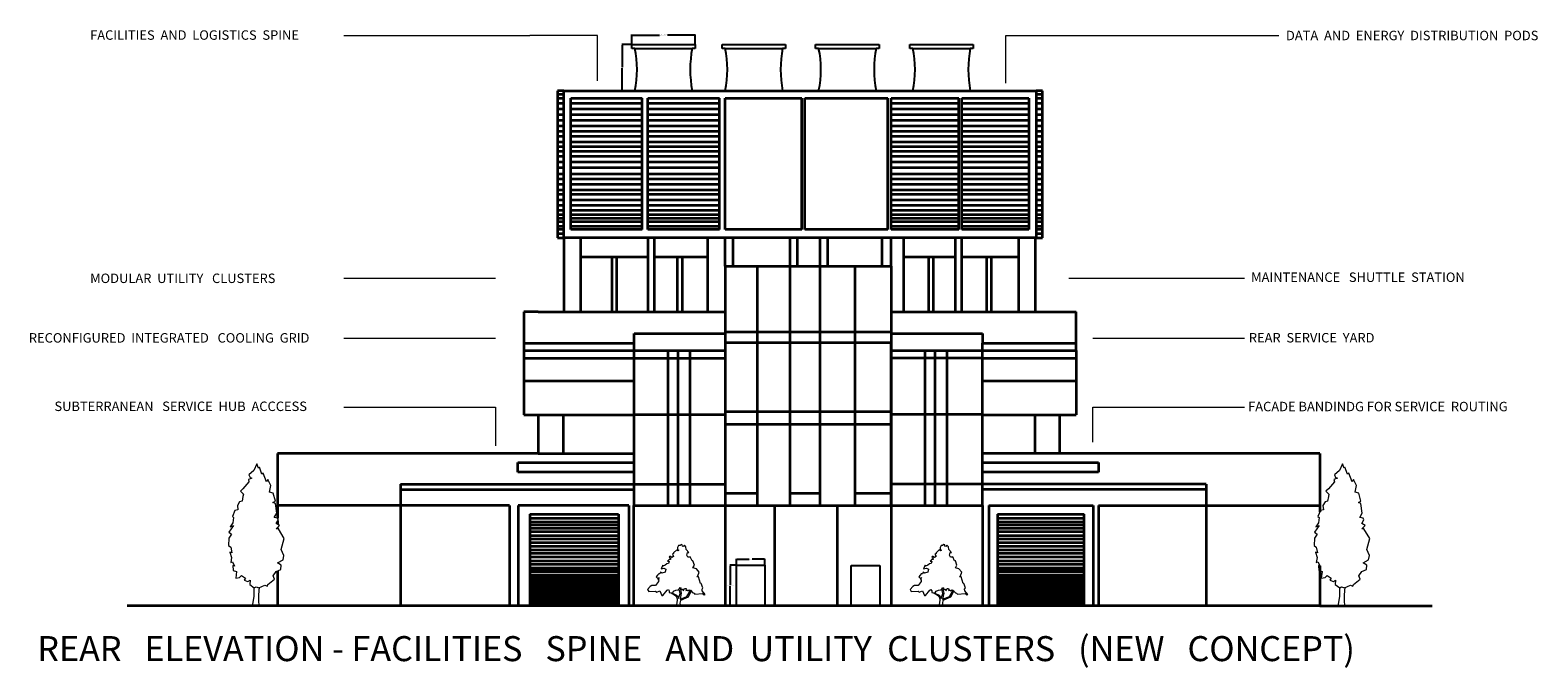
# Model space of a CAD drawing. Units: inches. Extents: x 13 to 584, y -20 to 222.
import ezdxf

# ---------------------------------------------------------------- set-up
doc = ezdxf.new("R2010")
doc.units = ezdxf.units.IN
doc.header["$MEASUREMENT"] = 0
for name, color, linetype, lineweight in [('A-ANNO-DIMS', 2, 'Continuous', 18), ('A-ANNO-SYMB', 2, 'Continuous', 18), ('A-ANNO-TEXT', 7, 'Continuous', 25), ('A-DOOR', 4, 'Continuous', 25), ('A-ELEV', 7, 'Continuous', 35), ('A-EQPM', 8, 'Continuous', 25), ('L-PLNT', 3, 'Continuous', 18)]:
    doc.layers.add(name, color=color, linetype=linetype, lineweight=lineweight)
doc.styles.get("Standard").update_dxf_attribs({"font": 'arial.ttf'})
doc.dimstyles.get("Standard").update_dxf_attribs({"dimtxt": 0.18, "dimasz": 0.18, "dimexe": 0.18, "dimexo": 0.0625, "dimgap": 0.09, "dimtad": 0, "dimtih": 1, "dimtoh": 1, "dimdec": 4, "dimzin": 0, "dimdsep": 46, "dimtxsty": 'Standard', "dimcen": 0.09, "dimadec": 0, "dimazin": 0, "dimtfac": 1, "dimtdec": 4, "dimtofl": 0, "dimtmove": 0, "dimatfit": 3, "dimfxl": 1, "dimtolj": 1, "dimtzin": 0, "dimarcsym": 0})

# ---------------------------------------------------------------- blocks, each defined once
blk = doc.blocks.new('*U2')
blk.add_lwpolyline([(-2.754, 191.699), (-6.78, 182.851), (-13.682, 176.953), (-11.956, 173.266), (-9.656, 172.529), (-14.257, 170.317), (-13.682, 167.368), (-21.733, 157.783), (-25.184, 154.834), (-21.158, 150.41), (-21.733, 147.461), (-22.884, 140.825), (-26.334, 140.087), (-29.21, 134.926), (-28.635, 129.028), (-32.661, 128.291), (-36.111, 120.18), (-34.386, 118.706), (-35.536, 111.333), (-38.987, 106.171), (-34.386, 107.646), (-40.712, 98.798), (-37.261, 95.849), (-40.712, 90.688), (-41.287, 80.366), (-38.412, 78.154), (-36.686, 70.781), (-39.562, 71.518), (-37.261, 64.145), (-38.412, 57.509), (-36.111, 58.247), (-33.236, 52.348), (-35.536, 53.086), (-34.961, 46.45), (-30.36, 44.975), (-31.51, 36.128), (-26.334, 36.865), (-23.459, 39.814), (-18.283, 36.128), (-20.008, 33.178), (-14.832, 31.704), (-11.956, 33.178), (-12.531, 27.28), (-6.205, 22.856), (-3.905, 24.331), (0.121, 22.856), (8.173, 26.543), (11.624, 25.068), (12.199, 27.28), (21.4, 34.653), (19.675, 39.077), (23.701, 44.975), (30.027, 47.924), (30.602, 53.823), (25.426, 56.772), (32.903, 61.196), (34.053, 67.094), (30.602, 75.205), (34.628, 89.951), (26.576, 103.222), (23.701, 103.222), (28.302, 107.646), (23.701, 110.595), (26.576, 115.756), (25.426, 117.968), (20.825, 118.706), (24.276, 124.604), (22.551, 137.876), (19.1, 139.35), (22.551, 140.825), (19.675, 151.884), (14.499, 153.359), (16.224, 162.207), (12.199, 170.317), (10.473, 167.368), (5.872, 179.165), (4.147, 177.69), (0.696, 187.275), (-0.454, 185.8)], close=True)
for points in [[(-6.813, 23.669), (-6.813, 11.669), (-8.627, 0)], [(0.387, 23.669), (-0.576, 13.271), (-0.576, 3.686), (0, 0)]]:
    blk.add_lwpolyline(points)
blk = doc.blocks.new('*U3')
for points in [[(22.0124, 137.721), (18.5475, 141.5624), (15.5282, 138.2446), (13.8028, 139.3505), (13.3714, 142.1153), (11.2148, 143.2214), (8.1954, 140.4564), (4.7447, 141.0094), (2.1567, 136.0326), (2.1567, 131.6088), (5.6074, 129.9499), (3.0193, 128.2909), (0.4313, 130.5029), (-6.9015, 123.3141), (-6.9015, 121.6552), (-9.9208, 119.9963), (-9.0581, 118.3373), (-6.9015, 115.0195), (-10.7835, 112.2546), (-14.6656, 115.0195), (-16.8222, 114.4665), (-17.6849, 112.2546), (-14.6656, 111.7016), (-14.2342, 107.2778), (-17.6065, 107.8307), (-21.5669, 103.9599), (-17.2536, 103.4069), (-18.9789, 97.8771), (-22.8609, 97.3241), (-27.1743, 94.5593), (-32.3504, 91.7944), (-32.7817, 94.0063), (-36.6638, 85.7116), (-29.7624, 87.3705), (-25.449, 84.6056), (-26.743, 77.9699), (-34.507, 75.205), (-37.9578, 77.4169), (-39.2518, 74.099), (-42.2711, 73.5461), (-44.8592, 70.2282), (-47.8786, 66.3574), (-43.9965, 63.0395), (-41.4085, 64.6985), (-44.3346, 59.8898), (-42.2089, 60.1377), (-42.5159, 55.7849), (-49.6039, 46.4502), (-58.2307, 45.8972), (-62.1127, 43.6853), (-68.5828, 36.4966), (-65.9947, 32.0727), (-50.0352, 32.6257), (-47.0159, 30.4138), (-39.6831, 33.7317), (-34.507, 22.6721), (-32.3504, 22.6721), (-22.4296, 34.8376), (-19.4102, 36.4966), (-17.2536, 33.7317), (-17.2536, 29.8608), (-13.8028, 28.7549), (-9.0581, 28.7549), (-7.3328, 32.6257), (-1.7254, 35.3906), (3.8821, 35.9436), (6.4701, 38.1555), (6.9014, 38.7085), (8.1954, 41.4734), (9.9208, 40.3674), (11.2148, 35.9436), (14.2341, 37.6025), (15.0968, 36.4966), (15.9595, 33.7317), (18.9789, 38.7085), (21.9982, 38.7085), (23.2922, 36.4966), (21.9982, 34.2847), (25.4489, 35.3906), (26.743, 33.7317), (29.7623, 35.9436), (32.7817, 34.8376), (38.8204, 28.7549), (41.4084, 27.6489), (43.5651, 25.437), (61.6813, 27.0959), (65.132, 23.7781), (67.7201, 24.884), (60.8186, 33.7317), (60.3873, 37.0495), (62.544, 40.3674), (58.662, 50.874), (56.5053, 50.874), (52.1919, 66.3574), (47.8785, 66.9103), (50.4665, 69.1222), (53.9172, 77.9699), (47.0158, 85.1586), (38.3891, 87.9235), (42.2711, 94.0063)], [(42.2711, 94.0063), (38.8204, 104.5129), (36.6637, 104.5129), (32.3503, 113.9135), (29.7623, 113.3605), (26.743, 113.3605), (24.5862, 117.7844), (25.8802, 123.8671), (29.331, 123.8671), (22.8609, 131.6088), (21.9982, 137.6916)], [(-9.9208, 28.2019), (0, 23.2251), (3.4507, 19.9072), (4.7447, 15.4834), (8.6267, 27.0959), (6.4701, 37.6025)], [(8.1954, 40.3674), (11.2148, 27.6489), (8.1954, 13.8245), (24.5862, 19.9072), (32.7817, 34.2847)], [(-12.9401, 28.7549), (-2.588, 22.1191), (0.8626, 17.6953), (1.7253, 11.6125), (0, 0)], [(34.5071, 33.1787), (27.1743, 18.2483), (9.0581, 10.5066), (7.7641, 3.8708), (8.1954, 0)]]:
    blk.add_lwpolyline(points)
blk = doc.blocks.new('COOLING-UNIT')
for p, q in [((0, 16.07), (0, 17.49)), ((0, 17.49), (24.03, 17.49)), ((24.03, 17.49), (24.03, 16.07)), ((1.14, 16.07), (0, 16.07)), ((1.14, 16.07), (22.88, 16.07)), ((24.03, 16.07), (22.88, 16.07))]:
    blk.add_line(p, q)
for centre, radius, start, end in [((-35.24, 8.04), 37.26, 347.5421, 12.4579), ((66.1, 8.04), 43.96, 169.4653, 190.5347)]:
    blk.add_arc(centre, radius, start, end)
blk = doc.blocks.new('DOOR-SERVICE')
for p, q in [((0, 0), (0, 15.29)), ((0, 15.29), (10.82, 15.29)), ((10.82, 15.29), (10.82, 0))]:
    blk.add_line(p, q)
blk = doc.blocks.new('*D6')
at = {"layer": 'A-ANNO-DIMS', "color": 0, "lineweight": -2, "transparency": 16777216}
for p, q in [((241.11, 216.34), (241.11, 220.06)), ((241.29, 219.88), (251.66, 219.88)), ((264.97, 219.88), (254.6, 219.88)), ((265.15, 216.34), (265.15, 220.06))]:
    blk.add_line(p, q, dxfattribs=at)
at = {"layer": 'A-ANNO-DIMS', "color": 0, "transparency": 16777216}
for points in [[(241.29, 219.91), (241.29, 219.85), (241.11, 219.88)], [(264.97, 219.91), (264.97, 219.85), (265.15, 219.88)]]:
    blk.add_solid(points, dxfattribs=at)
at = {"layer": 'Defpoints', "color": 0, "transparency": 16777216}
for p in [(265.15, 219.88), (241.11, 216.27), (265.15, 216.27)]:
    blk.add_point(p, dxfattribs=at)
at = {"layer": 'A-ANNO-DIMS', "color": 0, "transparency": 16777216, "insert": (253.13, 219.88), "char_height": 0.18, "attachment_point": 5}
blk.add_mtext('\\A1;COOLING UNIT 24 TYP.', dxfattribs=at)
blk = doc.blocks.new('*D7')
at = {"layer": 'A-ANNO-DIMS', "color": 0, "lineweight": -2, "transparency": 16777216}
for p, q in [((241.05, 216.27), (237.33, 216.27)), ((237.51, 216.09), (237.51, 207.71)), ((237.51, 198.96), (237.51, 207.35)), ((241.05, 198.78), (237.33, 198.78))]:
    blk.add_line(p, q, dxfattribs=at)
at = {"layer": 'A-ANNO-DIMS', "color": 0, "transparency": 16777216}
for points in [[(237.48, 216.09), (237.54, 216.09), (237.51, 216.27)], [(237.48, 198.96), (237.54, 198.96), (237.51, 198.78)]]:
    blk.add_solid(points, dxfattribs=at)
at = {"layer": 'Defpoints', "color": 0, "transparency": 16777216}
for p in [(237.51, 216.27), (241.11, 216.27), (241.11, 198.78)]:
    blk.add_point(p, dxfattribs=at)
at = {"layer": 'A-ANNO-DIMS', "color": 0, "transparency": 16777216, "insert": (237.51, 207.53), "char_height": 0.18, "attachment_point": 5}
blk.add_mtext('\\A1;17 TYP.', dxfattribs=at)
blk = doc.blocks.new('*D8')
at = {"layer": 'A-ANNO-DIMS', "color": 0, "lineweight": -2, "transparency": 16777216}
for p, q in [((280.67, 19.12), (278.26, 19.12)), ((278.44, 18.94), (278.44, 11.66)), ((278.44, 4.01), (278.44, 11.29)), ((280.67, 3.83), (278.26, 3.83))]:
    blk.add_line(p, q, dxfattribs=at)
at = {"layer": 'A-ANNO-DIMS', "color": 0, "transparency": 16777216}
for points in [[(278.41, 18.94), (278.47, 18.94), (278.44, 19.12)], [(278.41, 4.01), (278.47, 4.01), (278.44, 3.83)]]:
    blk.add_solid(points, dxfattribs=at)
at = {"layer": 'Defpoints', "color": 0, "transparency": 16777216}
for p in [(278.44, 19.12), (280.73, 19.12), (280.73, 3.83)]:
    blk.add_point(p, dxfattribs=at)
at = {"layer": 'A-ANNO-DIMS', "color": 0, "transparency": 16777216, "insert": (278.44, 11.47), "char_height": 0.18, "attachment_point": 5}
blk.add_mtext('\\A1;SERVICE DOOR 15 TYP.', dxfattribs=at)
blk = doc.blocks.new('*D9')
at = {"layer": 'A-ANNO-DIMS', "color": 0, "lineweight": -2, "transparency": 16777216}
for p, q in [((280.73, 19.18), (280.73, 21.59)), ((280.91, 21.41), (285.62, 21.41)), ((291.37, 21.41), (286.66, 21.41)), ((291.55, 19.18), (291.55, 21.59))]:
    blk.add_line(p, q, dxfattribs=at)
at = {"layer": 'A-ANNO-DIMS', "color": 0, "transparency": 16777216}
for points in [[(280.91, 21.44), (280.91, 21.38), (280.73, 21.41)], [(291.37, 21.44), (291.37, 21.38), (291.55, 21.41)]]:
    blk.add_solid(points, dxfattribs=at)
at = {"layer": 'Defpoints', "color": 0, "transparency": 16777216}
for p in [(280.73, 19.12), (291.55, 21.41), (291.55, 19.12)]:
    blk.add_point(p, dxfattribs=at)
at = {"layer": 'A-ANNO-DIMS', "color": 0, "transparency": 16777216, "insert": (286.14, 21.41), "char_height": 0.18, "attachment_point": 5}
blk.add_mtext('\\A1;11 TYP.', dxfattribs=at)

msp = doc.modelspace()

# ---------------------------------------------------------------- linework, layer by layer
at = {"layer": 'A-ANNO-SYMB'}
for p, q in [((132.16, 219.75), (202.59, 219.75)), ((228.21, 219.75), (202.59, 219.75)), ((228.21, 202.53), (228.21, 219.75)), ((382.77, 201.61), (382.77, 219.75)), ((382.77, 219.75), (486.08, 219.75)), ((132.16, 127.9), (189.57, 127.9)), ((406.56, 127.9), (473.06, 127.9)), ((132.16, 105.07), (189.57, 105.07)), ((415.65, 105.07), (473.06, 105.07)), ((132.16, 78.99), (189.57, 78.99)), ((189.57, 78.99), (189.57, 64.36)), ((415.65, 65.75), (415.65, 78.99)), ((415.65, 78.99), (473.06, 78.99))]:
    msp.add_line(p, q, dxfattribs=at)
at = {"layer": 'A-ELEV'}
for p, q in [((215.46, 198.78), (213.08, 198.78)), ((213.08, 198.78), (213.08, 143.13)), ((213.08, 197.55), (215.46, 197.55)), ((213.08, 195.94), (215.46, 195.94)), ((213.08, 194.05), (215.46, 194.05)), ((215.46, 198.78), (394.39, 198.78)), ((215.46, 143.13), (215.46, 198.78)), ((218.09, 195.94), (245.06, 195.94)), ((218.09, 146.31), (218.09, 195.94)), ((218.09, 194.05), (245.06, 194.05)), ((245.06, 146.31), (245.06, 195.94)), ((247.21, 195.94), (274.37, 195.94)), ((247.21, 146.31), (247.21, 195.94)), ((247.21, 194.05), (274.37, 194.05)), ((274.37, 146.31), (274.37, 195.94)), ((276.52, 195.94), (305.52, 195.94)), ((276.52, 146.31), (276.52, 195.94)), ((305.52, 146.31), (305.52, 195.94)), ((306.69, 195.94), (338.12, 195.94)), ((306.69, 146.31), (306.69, 195.94)), ((338.12, 146.31), (338.12, 195.94)), ((339.29, 195.94), (364.89, 195.94)), ((339.29, 146.31), (339.29, 195.94)), ((339.29, 194.05), (364.89, 194.05)), ((364.89, 146.31), (364.89, 195.94)), ((366.07, 195.94), (391.39, 195.94)), ((366.07, 146.31), (366.07, 195.94)), ((366.07, 194.05), (391.39, 194.05)), ((391.39, 195.94), (391.39, 146.31)), ((396.59, 198.78), (394.21, 198.78)), ((394.21, 198.78), (394.21, 143.13)), ((394.21, 197.55), (396.59, 197.55)), ((394.21, 195.94), (396.59, 195.94)), ((394.21, 194.05), (396.59, 194.05)), ((396.59, 143.13), (396.59, 198.78)), ((213.08, 191.91), (215.46, 191.91)), ((213.08, 189.77), (215.46, 189.77)), ((218.09, 191.91), (245.06, 191.91)), ((218.09, 189.77), (245.06, 189.77)), ((247.21, 191.91), (274.37, 191.91)), ((247.21, 189.77), (274.37, 189.77)), ((339.29, 191.91), (364.89, 191.91)), ((339.29, 189.77), (364.89, 189.77)), ((366.07, 191.91), (391.39, 191.91)), ((366.07, 189.77), (391.39, 189.77)), ((394.21, 191.91), (396.59, 191.91)), ((394.21, 189.77), (396.59, 189.77)), ((213.08, 187.63), (215.46, 187.63)), ((213.08, 185.49), (215.46, 185.49)), ((213.08, 183.54), (215.46, 183.54)), ((218.09, 187.63), (245.06, 187.63)), ((218.09, 185.49), (245.06, 185.49)), ((218.09, 183.54), (245.06, 183.54)), ((247.21, 187.63), (274.37, 187.63)), ((247.21, 185.49), (274.37, 185.49)), ((247.21, 183.54), (274.37, 183.54)), ((339.29, 187.63), (364.89, 187.63)), ((339.29, 185.49), (364.89, 185.49)), ((339.29, 183.54), (364.89, 183.54)), ((366.07, 187.63), (391.39, 187.63)), ((366.07, 185.49), (391.39, 185.49)), ((366.07, 183.54), (391.39, 183.54)), ((394.21, 187.63), (396.59, 187.63)), ((394.21, 185.49), (396.59, 185.49)), ((394.21, 183.54), (396.59, 183.54)), ((213.08, 181.6), (215.46, 181.6)), ((213.08, 179.46), (215.46, 179.46)), ((213.08, 177.71), (215.46, 177.71)), ((218.09, 181.6), (245.06, 181.6)), ((218.09, 179.46), (245.06, 179.46)), ((218.09, 177.71), (245.06, 177.71)), ((247.21, 181.6), (274.37, 181.6)), ((247.21, 179.46), (274.37, 179.46)), ((247.21, 177.71), (274.37, 177.71)), ((339.29, 181.6), (364.89, 181.6)), ((339.29, 179.46), (364.89, 179.46)), ((339.29, 177.71), (364.89, 177.71)), ((366.07, 181.6), (391.39, 181.6)), ((366.07, 179.46), (391.39, 179.46)), ((366.07, 177.71), (391.39, 177.71)), ((394.21, 181.6), (396.59, 181.6)), ((394.21, 179.46), (396.59, 179.46)), ((394.21, 177.71), (396.59, 177.71)), ((213.08, 175.96), (215.46, 175.96)), ((213.08, 174.01), (215.46, 174.01)), ((213.08, 171.85), (215.46, 171.85)), ((218.09, 175.96), (245.06, 175.96)), ((218.09, 174.01), (245.06, 174.01)), ((218.09, 171.85), (245.06, 171.85)), ((247.21, 175.96), (274.37, 175.96)), ((247.21, 174.01), (274.37, 174.01)), ((247.21, 171.85), (274.37, 171.85)), ((339.29, 175.96), (364.89, 175.96)), ((339.29, 174.01), (364.89, 174.01)), ((339.29, 171.85), (364.89, 171.85)), ((366.07, 175.96), (391.39, 175.96)), ((366.07, 174.01), (391.39, 174.01)), ((366.07, 171.85), (391.39, 171.85)), ((394.21, 175.96), (396.59, 175.96)), ((394.21, 174.01), (396.59, 174.01)), ((394.21, 171.85), (396.59, 171.85)), ((213.08, 169.71), (215.46, 169.71)), ((213.08, 167.37), (215.46, 167.37)), ((218.09, 169.71), (245.06, 169.71)), ((218.09, 167.37), (245.06, 167.37)), ((247.21, 169.71), (274.37, 169.71)), ((247.21, 167.37), (274.37, 167.37)), ((339.29, 169.71), (364.89, 169.71)), ((339.29, 167.37), (364.89, 167.37)), ((366.07, 169.71), (391.39, 169.71)), ((366.07, 167.37), (391.39, 167.37)), ((394.21, 169.71), (396.59, 169.71)), ((394.21, 167.37), (396.59, 167.37)), ((213.08, 165.43), (215.46, 165.43)), ((213.08, 163.48), (215.46, 163.48)), ((213.08, 161.34), (215.46, 161.34)), ((218.09, 165.43), (245.06, 165.43)), ((218.09, 163.48), (245.06, 163.48)), ((218.09, 161.34), (245.06, 161.34)), ((247.21, 165.43), (274.37, 165.43)), ((247.21, 163.48), (274.37, 163.48)), ((247.21, 161.34), (274.37, 161.34)), ((339.29, 165.43), (364.89, 165.43)), ((339.29, 163.48), (364.89, 163.48)), ((339.29, 161.34), (364.89, 161.34)), ((366.07, 165.43), (391.39, 165.43)), ((366.07, 163.48), (391.39, 163.48)), ((366.07, 161.34), (391.39, 161.34)), ((394.21, 165.43), (396.59, 165.43)), ((394.21, 163.48), (396.59, 163.48)), ((394.21, 161.34), (396.59, 161.34)), ((213.08, 159.59), (215.46, 159.59)), ((213.08, 157.45), (215.46, 157.45)), ((213.08, 155.51), (215.46, 155.51)), ((218.09, 159.59), (245.06, 159.59)), ((218.09, 157.45), (245.06, 157.45)), ((218.09, 155.51), (245.06, 155.51)), ((247.21, 159.59), (274.37, 159.59)), ((247.21, 157.45), (274.37, 157.45)), ((247.21, 155.51), (274.37, 155.51)), ((339.29, 159.59), (364.89, 159.59)), ((339.29, 157.45), (364.89, 157.45)), ((339.29, 155.51), (364.89, 155.51)), ((366.07, 159.59), (391.39, 159.59)), ((366.07, 157.45), (391.39, 157.45)), ((366.07, 155.51), (391.39, 155.51)), ((394.21, 159.59), (396.59, 159.59)), ((394.21, 157.45), (396.59, 157.45)), ((394.21, 155.51), (396.59, 155.51)), ((213.08, 153.53), (215.46, 153.53)), ((213.08, 151.97), (215.46, 151.97)), ((213.08, 150.61), (215.46, 150.61)), ((213.08, 149.25), (215.46, 149.25)), ((218.09, 153.53), (245.06, 153.53)), ((218.09, 151.97), (245.06, 151.97)), ((218.09, 150.61), (245.06, 150.61)), ((218.09, 149.25), (245.06, 149.25)), ((247.21, 153.53), (274.37, 153.53)), ((247.21, 151.97), (274.37, 151.97)), ((247.21, 150.61), (274.37, 150.61)), ((247.21, 149.25), (274.37, 149.25)), ((339.29, 153.53), (364.89, 153.53)), ((339.29, 151.97), (364.89, 151.97)), ((339.29, 150.61), (364.89, 150.61)), ((339.29, 149.25), (364.89, 149.25)), ((366.07, 153.53), (391.39, 153.53)), ((366.07, 151.97), (391.39, 151.97)), ((366.07, 150.61), (391.39, 150.61)), ((366.07, 149.25), (391.39, 149.25)), ((394.21, 153.53), (396.59, 153.53)), ((394.21, 151.97), (396.59, 151.97)), ((394.21, 150.61), (396.59, 150.61)), ((394.21, 149.25), (396.59, 149.25)), ((213.08, 147.5), (215.46, 147.5)), ((215.46, 146.31), (213.08, 146.31)), ((213.08, 144.72), (215.46, 144.72)), ((213.08, 143.13), (215.46, 143.13)), ((394.39, 143.13), (215.46, 143.13)), ((215.46, 143.13), (215.46, 115.06)), ((218.09, 147.5), (245.06, 147.5)), ((245.06, 146.31), (218.09, 146.31)), ((221.89, 115.06), (221.89, 143.13)), ((247.21, 147.5), (274.37, 147.5)), ((274.37, 146.31), (247.21, 146.31)), ((247.33, 115.06), (247.33, 143.13)), ((249.68, 115.06), (249.68, 143.13)), ((269.94, 115.06), (269.94, 143.13)), ((305.52, 146.31), (276.52, 146.31)), ((276.52, 132.43), (276.52, 143.13)), ((279.57, 132.43), (279.57, 143.13)), ((301.14, 132.43), (301.14, 143.13)), ((303.82, 132.43), (303.82, 143.13)), ((338.12, 146.31), (306.69, 146.31)), ((312.4, 132.43), (312.4, 143.13)), ((315.34, 132.43), (315.34, 143.13)), ((335.95, 132.43), (335.95, 143.13)), ((339.29, 147.5), (364.89, 147.5)), ((364.89, 146.31), (339.29, 146.31)), ((339.29, 132.43), (339.29, 143.13)), ((344.15, 115.06), (344.15, 143.13)), ((363.7, 115.06), (363.7, 143.13)), ((366.06, 115.06), (366.06, 143.13)), ((366.07, 147.5), (391.39, 147.5)), ((391.39, 146.31), (366.07, 146.31)), ((387.46, 143.13), (387.46, 115.06)), ((393.89, 115.06), (393.89, 143.13)), ((394.21, 147.5), (396.59, 147.5)), ((396.59, 146.31), (394.21, 146.31)), ((394.21, 144.72), (396.59, 144.72)), ((394.21, 143.13), (396.59, 143.13)), ((221.89, 135.96), (247.33, 135.96)), ((233.69, 115.06), (233.69, 135.96)), ((235.54, 115.06), (235.54, 135.96)), ((249.68, 135.96), (269.94, 135.96)), ((258.47, 115.06), (258.47, 135.96)), ((260.31, 115.06), (260.31, 135.96)), ((276.52, 132.43), (339.29, 132.43)), ((276.52, 132.43), (276.52, 41.71)), ((288.58, 132.43), (288.58, 41.71)), ((301.02, 132.43), (301.02, 41.71)), ((312.33, 132.43), (312.33, 41.71)), ((325.52, 132.43), (325.52, 41.71)), ((339.29, 132.43), (339.29, 41.71)), ((344.15, 135.96), (363.7, 135.96)), ((353.55, 115.06), (353.55, 135.96)), ((355.39, 115.06), (355.39, 135.96)), ((366.06, 135.96), (387.46, 135.96)), ((375.49, 115.06), (375.49, 135.96)), ((377.33, 115.06), (377.33, 135.96)), ((205.68, 115.06), (200.31, 115.06)), ((200.31, 115.06), (200.31, 103.27)), ((205.68, 115.06), (276.52, 115.06)), ((339.29, 115.06), (409.32, 115.06)), ((409.32, 103.27), (409.32, 115.06)), ((200.31, 103.27), (241.99, 103.27)), ((200.31, 103.27), (200.31, 100.49)), ((241.99, 103.27), (241.99, 106.83)), ((241.99, 106.83), (276.52, 106.83)), ((241.99, 41.71), (241.99, 103.27)), ((276.52, 107.58), (339.29, 107.58)), ((276.52, 103.44), (339.29, 103.44)), ((339.29, 106.83), (373.83, 106.83)), ((339.29, 103.27), (339.29, 103.27)), ((339.29, 41.71), (339.29, 103.27)), ((373.83, 106.83), (373.83, 103.27)), ((373.83, 103.27), (409.32, 103.27)), ((373.83, 41.71), (373.83, 103.27)), ((409.32, 100.49), (409.32, 103.27)), ((200.31, 100.49), (276.52, 100.49)), ((200.31, 100.49), (200.31, 76.14)), ((200.31, 97.54), (241.99, 97.54)), ((241.99, 97.54), (276.52, 97.54)), ((254.94, 41.71), (254.94, 100.49)), ((258.69, 41.71), (258.69, 100.49)), ((263.29, 41.71), (263.29, 100.49)), ((339.29, 100.49), (409.32, 100.49)), ((339.29, 97.54), (339.29, 97.54)), ((373.83, 97.54), (339.29, 97.54)), ((352.21, 41.71), (352.21, 100.49)), ((355.96, 41.71), (355.96, 100.49)), ((360.56, 41.71), (360.56, 100.49)), ((373.83, 97.54), (409.32, 97.54)), ((409.32, 100.49), (409.32, 76.14)), ((200.31, 88.93), (241.99, 88.93)), ((339.29, 88.93), (339.29, 88.93)), ((373.83, 88.93), (409.32, 88.93)), ((200.31, 76.14), (241.99, 76.14)), ((205.75, 76.14), (205.75, 61.41)), ((215.12, 76.14), (215.12, 61.41)), ((241.99, 76.27), (276.52, 76.27)), ((276.52, 77.4), (339.29, 77.4)), ((373.83, 76.27), (339.29, 76.27)), ((339.29, 76.14), (339.29, 76.14)), ((373.83, 76.14), (409.32, 76.14)), ((393.73, 76.14), (393.73, 61.41)), ((403.1, 76.14), (403.1, 61.41)), ((276.52, 72.51), (339.29, 72.51)), ((205.75, 61.41), (107.03, 61.41)), ((107.03, 61.41), (107.03, 37.01)), ((197.95, 58.07), (241.96, 58.07)), ((197.95, 54.42), (197.95, 58.07)), ((205.75, 61.41), (241.99, 61.41)), ((403.1, 61.41), (373.83, 61.41)), ((373.83, 58.07), (417.83, 58.07)), ((501.6, 61.41), (402.88, 61.41)), ((417.83, 58.07), (417.83, 54.42)), ((501.6, 61.41), (501.6, 39.36)), ((241.96, 54.42), (197.95, 54.42)), ((417.83, 54.42), (373.83, 54.42)), ((153.64, 49.86), (153.64, 3.81)), ((153.64, 49.86), (241.99, 49.86)), ((153.64, 47.85), (241.99, 47.85)), ((241.99, 49.86), (276.52, 49.86)), ((276.52, 46.49), (288.58, 46.49)), ((301.02, 46.49), (312.33, 46.49)), ((325.52, 46.49), (339.29, 46.49)), ((373.83, 49.86), (339.29, 49.86)), ((458.5, 49.86), (373.83, 49.86)), ((458.5, 47.85), (373.83, 47.85)), ((458.5, 49.86), (458.5, 3.81)), ((153.64, 41.71), (107.03, 41.71)), ((194.9, 41.71), (153.64, 41.71)), ((194.9, 41.71), (194.9, 3.81)), ((240.08, 41.71), (198.15, 41.71)), ((198.15, 41.71), (198.15, 3.81)), ((240.08, 41.71), (240.08, 3.81)), ((241.99, 41.71), (241.83, 41.71)), ((241.83, 41.71), (241.83, 3.81)), ((241.99, 41.71), (276.52, 41.71)), ((276.49, 41.71), (276.49, 3.81)), ((276.52, 41.71), (339.29, 41.71)), ((295.1, 41.71), (295.1, 3.81)), ((318.94, 41.71), (318.94, 3.81)), ((339.29, 41.71), (373.83, 41.71)), ((339.3, 41.71), (339.3, 3.81)), ((373.83, 41.71), (373.93, 41.71)), ((373.93, 41.71), (373.93, 3.81)), ((376.25, 41.71), (415.8, 41.71)), ((376.25, 41.71), (376.25, 3.81)), ((415.8, 41.71), (415.8, 3.81)), ((417.83, 41.71), (458.5, 41.71)), ((417.83, 41.71), (417.83, 3.81)), ((458.5, 41.71), (501.6, 41.71)), ((107.03, 35.81), (107.03, 34.66)), ((202.49, 38.48), (230.93, 38.48)), ((202.49, 38.48), (202.49, 3.81)), ((202.49, 36.92), (236.09, 36.92)), ((202.49, 35.63), (236.09, 35.63)), ((202.49, 34.46), (236.09, 34.46)), ((230.93, 38.48), (236.09, 38.48)), ((236.09, 38.48), (236.09, 3.81)), ((276.49, 38.48), (276.52, 38.48)), ((379.63, 38.48), (412.34, 38.48)), ((379.63, 38.48), (379.63, 3.81)), ((379.63, 36.92), (412.34, 36.92)), ((379.63, 35.63), (412.34, 35.63)), ((379.63, 34.46), (412.34, 34.46)), ((412.34, 3.81), (412.34, 38.48)), ((107.03, 33.37), (107.03, 32.92)), ((202.49, 33.16), (236.09, 33.16)), ((202.49, 31.87), (236.09, 31.87)), ((202.49, 30.44), (236.09, 30.44)), ((202.49, 29.15), (236.09, 29.15)), ((379.63, 33.16), (412.34, 33.16)), ((379.63, 31.87), (412.34, 31.87)), ((379.63, 30.44), (412.34, 30.44)), ((379.63, 29.15), (412.34, 29.15)), ((202.49, 27.72), (236.09, 27.72)), ((202.49, 26.43), (236.09, 26.43)), ((202.49, 25), (236.09, 25)), ((202.49, 23.71), (236.09, 23.71)), ((379.63, 27.72), (412.34, 27.72)), ((379.63, 26.43), (412.34, 26.43)), ((379.63, 25), (412.34, 25)), ((379.63, 23.71), (412.34, 23.71)), ((202.49, 22.28), (236.09, 22.28)), ((202.49, 20.86), (236.09, 20.86)), ((202.49, 19.56), (236.09, 19.56)), ((202.49, 18.14), (236.09, 18.14)), ((202.49, 17.53), (236.09, 17.53)), ((379.63, 22.28), (412.34, 22.28)), ((379.63, 20.86), (412.34, 20.86)), ((379.63, 19.56), (412.34, 19.56)), ((379.63, 18.14), (412.34, 18.14)), ((379.63, 17.53), (412.34, 17.53)), ((501.6, 18.91), (501.6, 3.81)), ((107.03, 16.96), (107.03, 3.81)), ((202.49, 16.84), (236.09, 16.84)), ((202.49, 15.55), (236.09, 15.55)), ((202.49, 14.89), (236.09, 14.89)), ((202.49, 14.1), (236.09, 14.1)), ((202.49, 13.36), (236.09, 13.36)), ((202.49, 12.54), (236.09, 12.54)), ((202.49, 11.5), (236.09, 11.5)), ((379.63, 16.84), (412.34, 16.84)), ((379.63, 15.55), (412.34, 15.55)), ((379.63, 14.89), (412.34, 14.89)), ((379.63, 14.1), (412.34, 14.1)), ((379.63, 13.36), (412.34, 13.36)), ((379.63, 12.54), (412.34, 12.54)), ((379.63, 11.5), (412.34, 11.5)), ((202.49, 10.47), (236.09, 10.47)), ((202.49, 9.43), (236.09, 9.43)), ((202.49, 8.53), (236.09, 8.53)), ((202.49, 7.62), (236.09, 7.62)), ((202.49, 6.71), (236.09, 6.71)), ((202.49, 5.93), (236.09, 5.93)), ((379.63, 10.47), (412.34, 10.47)), ((379.63, 9.43), (412.34, 9.43)), ((379.63, 8.53), (412.34, 8.53)), ((379.63, 7.62), (412.34, 7.62)), ((379.63, 6.71), (412.34, 6.71)), ((379.63, 5.93), (412.34, 5.93)), ((107.03, 3.81), (50.19, 3.81)), ((501.6, 3.81), (107.03, 3.81)), ((202.49, 4.9), (236.09, 4.9)), ((379.63, 4.9), (412.34, 4.9)), ((501.6, 3.81), (544.16, 3.81))]:
    msp.add_line(p, q, dxfattribs=at)

# ---------------------------------------------------------------- block references
at = {"layer": 'A-DOOR'}
for p in [(280.73, 3.83), (324.21, 3.81)]:
    msp.add_blockref('DOOR-SERVICE', p, dxfattribs=at)
at = {"layer": 'A-EQPM'}
for p in [(241.11, 198.78), (275.32, 198.78), (310.73, 198.78), (346.37, 198.78)]:
    msp.add_blockref('COOLING-UNIT', p, dxfattribs=at)
at = {"layer": 'L-PLNT'}
for name, p, xscale, yscale, zscale in [('*U2', (99.98, 4.25), 0.2777393630674211, 0.2777393630674211, 0.2777393630674211), ('*U2', (510.89, 4.25), 0.2777393630674211, 0.2777393630674211, 0.2777393630674211), ('*U3', (258.08, 4.12), 0.1598369605741295, 0.1598369605741295, 0.1598369605741295), ('*U3', (357.48, 4.12), 0.1598369605741295, 0.1598369605741295, 0.1598369605741295)]:
    msp.add_blockref(name, p, dxfattribs=dict(at, xscale=xscale, yscale=yscale, zscale=zscale))

# ---------------------------------------------------------------- texts
at = {"layer": 'A-ANNO-TEXT'}
for s, height, p in [('FACILITIES  AND  LOGISTICS  SPINE', 3.5792, (36.11, 218.1)), ('DATA  AND  ENERGY  DISTRIBUTION  PODS', 3.5792, (488.76, 217.93)), ('MODULAR  UTILITY   CLUSTERS', 3.5792, (36.11, 126)), ('MAINTENANCE   SHUTTLE  STATION', 3.5792, (475.57, 126.41)), ('RECONFIGURED  INTEGRATED   COOLING  GRID  ', 3.5792, (12.91, 103.45)), ('REAR  SERVICE  YARD', 3.5792, (474.71, 103.5)), ('SUBTERRANEAN   SERVICE  HUB  ACCCESS', 3.5792, (22.6, 77.54)), ('FACADE BANDINDG FOR SERVICE  ROUTING', 3.5792, (474.43, 77.45)), ('REAR   ELEVATION - FACILITIES   SPINE   AND  UTILITY  CLUSTERS   (NEW   CONCEPT)   ', 9.4809, (16.1, -17.16))]:
    msp.add_text(s, height=height, dxfattribs=at).set_placement(p)

# ---------------------------------------------------------------- dimensions: what is measured, and where the dimension line sits
at = {"layer": 'A-ANNO-DIMS'}
for base, p1, p2, text, picture, middle in [((265.15, 219.88), (241.11, 216.27), (265.15, 216.27), 'COOLING UNIT <> TYP.', '*D6', (253.13, 219.88)), ((291.55, 21.41), (280.73, 19.12), (291.55, 19.12), '<> TYP.', '*D9', (286.14, 21.41))]:
    dim = msp.add_linear_dim(base=base, p1=p1, p2=p2, text=text, dimstyle='Standard', override={"dimdec": 0, "dimlfac": 1, "dimrnd": 0, "dimzin": 0, "dimdsep": 46, "dimlunit": 2}, dxfattribs=at)
    dim.commit()
    dim.dimension.update_dxf_attribs({"geometry": picture, "text_midpoint": middle})
for base, p1, p2, text, picture, middle in [((237.51, 216.27), (241.11, 198.78), (241.11, 216.27), '<> TYP.', '*D7', (237.51, 207.53)), ((278.44, 19.12), (280.73, 3.83), (280.73, 19.12), 'SERVICE DOOR <> TYP.', '*D8', (278.44, 11.47))]:
    dim = msp.add_linear_dim(base=base, p1=p1, p2=p2, angle=90, text=text, dimstyle='Standard', override={"dimdec": 0, "dimlfac": 1, "dimrnd": 0, "dimzin": 0, "dimdsep": 46, "dimlunit": 2}, dxfattribs=at)
    dim.commit()
    dim.dimension.update_dxf_attribs({"geometry": picture, "text_midpoint": middle})

doc.saveas('drawing.dxf')
